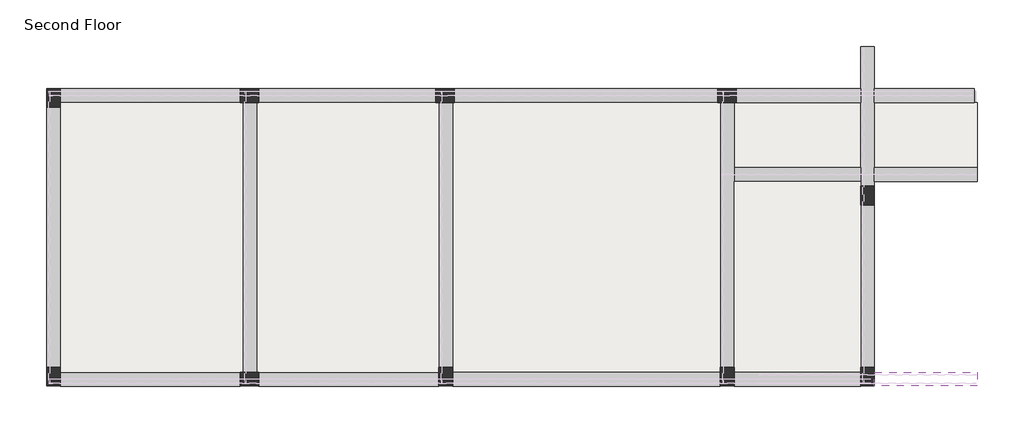
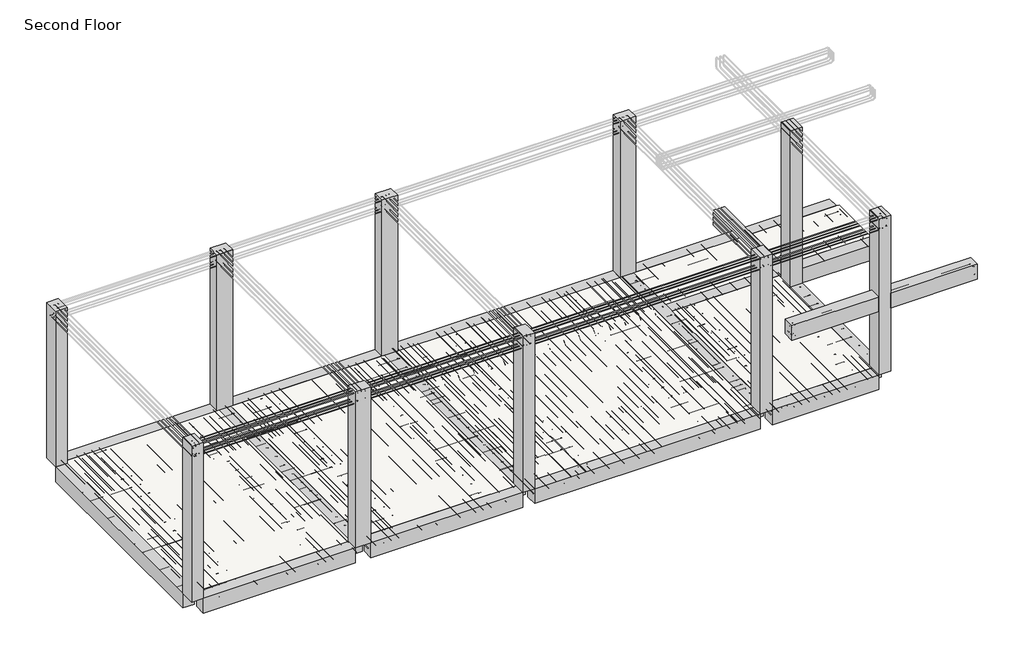
# One storey, part 1 of 4: 10 columns, 9 beams, 5 slabs.
"""IFC4 building model written with IfcOpenShell, lengths in millimetres."""

from ifc_helpers import new_model, si_unit, frame, origin, place, context, project, spatial, polyline, outline, extrude, faceted_brep, element, save

model = new_model("IFC4")

# Units and contexts
model_context = context("Model", 3, world=origin())
ifc_project = project(units=[si_unit("LENGTHUNIT", "METRE", prefix="MILLI")], contexts=[model_context])

# Site, building, storey
site = spatial("IfcSite", under=ifc_project)
building = spatial("IfcBuilding", under=site)
storey = spatial("IfcBuildingStorey", under=building, Name="Second Floor", Elevation=6400.8)

# Beams
placement = place(None, origin())
element("IfcBeam", 1, ObjectType="M_Concrete-Rectangular Beam : 9\" X12\"", at=placement, inside=storey, context=model_context, shape_type="Brep", body=[
    faceted_brep([(3956.0882476, 186.4334631, 6400.8), (3956.0882476, 415.0334631, 6400.8), (1885.9882476, 415.0334631, 6400.8), (1885.9882476, 186.4334631, 6400.8), (3956.0882476, 186.4334631, 6096.0), (1885.9882476, 186.4334631, 6096.0), (3956.0882476, 415.0334631, 6096.0), (1885.9882476, 415.0334631, 6096.0), (3956.0882476, 415.0334631, 6248.4), (1885.9882476, 415.0334631, 6248.4)], [[[0, 1, 2, 3]], [[4, 0, 3, 5]], [[6, 4, 5, 7]], [[1, 8, 6, 7, 9, 2]], [[1, 0, 4, 6, 8]], [[3, 2, 9, 7, 5]]]),
    faceted_brep([(-9150.3117524, 186.4334631, 6400.8), (-9150.3117524, 415.0334631, 6400.8), (-9150.3117524, 415.0334631, 6248.4), (-9150.3117524, 415.0334631, 6096.0), (-9150.3117524, 186.4334631, 6096.0), (-6203.9117524, 415.0334631, 6400.8), (-6203.9117524, 186.4334631, 6400.8), (-6203.9117524, 186.4334631, 6096.0), (-6203.9117524, 415.0334631, 6096.0)], [[[0, 1, 2, 3, 4]], [[5, 6, 7, 8]], [[1, 0, 6, 5]], [[0, 4, 7, 6]], [[4, 3, 8, 7]], [[3, 2, 1, 5, 8]]]),
    faceted_brep([(-5899.1117524, 186.4334631, 6400.8), (-5899.1117524, 415.0334631, 6400.8), (-5899.1117524, 415.0334631, 6096.0), (-5899.1117524, 186.4334631, 6096.0), (-2952.7117524, 415.0334631, 6400.8), (-2952.7117524, 186.4334631, 6400.8), (-2952.7117524, 186.4334631, 6096.0), (-2952.7117524, 415.0334631, 6096.0), (-2952.7117524, 415.0334631, 6248.4)], [[[0, 1, 2, 3]], [[4, 5, 6, 7, 8]], [[1, 0, 5, 4]], [[0, 3, 6, 5]], [[3, 2, 7, 6]], [[2, 1, 4, 8, 7]]]),
    faceted_brep([(-2724.1117524, 186.4334631, 6400.8), (-2724.1117524, 415.0334631, 6400.8), (-2724.1117524, 415.0334631, 6248.4), (-2724.1117524, 415.0334631, 6096.0), (-2724.1117524, 186.4334631, 6096.0), (1657.3882476, 415.0334631, 6400.8), (1657.3882476, 186.4334631, 6400.8), (1657.3882476, 186.4334631, 6096.0), (1657.3882476, 415.0334631, 6096.0), (1657.3882476, 415.0334631, 6248.4)], [[[0, 1, 2, 3, 4]], [[5, 6, 7, 8, 9]], [[1, 0, 6, 5]], [[0, 4, 7, 6]], [[4, 3, 8, 7]], [[3, 2, 1, 5, 9, 8]]]),
])
element("IfcBeam", 2, ObjectType="M_Concrete-Rectangular Beam : 9\" X12\"", at=placement, inside=storey, context=model_context, shape_type="Brep", body=[
    faceted_brep([(3956.0882476, 5755.7334631, 6400.8), (4184.6882476, 5755.7334631, 6400.8), (4184.6882476, 5755.7334631, 6096.0), (3956.0882476, 5755.7334631, 6096.0), (3956.0882476, 5063.2334631, 6400.8), (3956.0882476, 4834.6334631, 6400.8), (3956.0882476, 3767.8334631, 6400.8), (3956.0882476, 3539.2334631, 6400.8), (3956.0882476, 3463.0334631, 6400.8), (4184.6882476, 3463.0334631, 6400.8), (4184.6882476, 3539.2334631, 6400.8), (4184.6882476, 3767.8334631, 6400.8), (4184.6882476, 4834.6334631, 6400.8), (4184.6882476, 5063.2334631, 6400.8), (4184.6882476, 3463.0334631, 6096.0), (4184.6882476, 3539.2334631, 6096.0), (4184.6882476, 3767.8334631, 6096.0), (4184.6882476, 4834.6334631, 6096.0), (4184.6882476, 5063.2334631, 6096.0), (3956.0882476, 3463.0334631, 6096.0), (3956.0882476, 3539.2334631, 6096.0), (3956.0882476, 3767.8334631, 6096.0), (3956.0882476, 4834.6334631, 6096.0), (3956.0882476, 5063.2334631, 6096.0)], [[[0, 1, 2, 3]], [[1, 0, 4, 5, 6, 7, 8, 9, 10, 11, 12, 13]], [[2, 1, 13, 12, 11, 10, 9, 14, 15, 16, 17, 18]], [[3, 2, 18, 17, 16, 15, 14, 19, 20, 21, 22, 23]], [[0, 3, 23, 22, 21, 20, 19, 8, 7, 6, 5, 4]], [[9, 8, 19, 14]]]),
    faceted_brep([(4184.6882476, 491.2334631, 6400.8), (3956.0882476, 491.2334631, 6400.8), (3956.0882476, 491.2334631, 6096.0), (4184.6882476, 491.2334631, 6096.0), (3956.0882476, 3158.2334631, 6400.8), (4184.6882476, 3158.2334631, 6400.8), (4184.6882476, 3158.2334631, 6096.0), (3956.0882476, 3158.2334631, 6096.0)], [[[0, 1, 2, 3]], [[4, 5, 6, 7]], [[1, 0, 5, 4]], [[0, 3, 6, 5]], [[3, 2, 7, 6]], [[2, 1, 4, 7]]]),
])
element("IfcBeam", 3, ObjectType="M_Concrete-Rectangular Beam : 9\" X12\"", at=placement, inside=storey, context=model_context, shape_type="Brep", body=[
    faceted_brep([(5815.3882476, 4834.6334631, 6400.8), (5815.3882476, 4834.6334631, 6096.0), (5815.3882476, 5063.2334631, 6096.0), (5815.3882476, 5063.2334631, 6400.8), (4184.6882476, 4834.6334631, 6400.8), (4184.6882476, 5063.2334631, 6400.8), (4184.6882476, 5063.2334631, 6096.0), (4184.6882476, 4834.6334631, 6096.0), (4184.6882476, 4834.6334631, 6248.4)], [[[0, 1, 2, 3]], [[4, 5, 6, 7, 8]], [[0, 3, 5, 4]], [[3, 2, 6, 5]], [[2, 1, 7, 6]], [[1, 0, 4, 8, 7]]]),
    faceted_brep([(3956.0882476, 4834.6334631, 6400.8), (3956.0882476, 5063.2334631, 6400.8), (1924.0882476, 5063.2334631, 6400.8), (1924.0882476, 4834.6334631, 6400.8), (1924.0882476, 5063.2334631, 6096.0), (3956.0882476, 5063.2334631, 6096.0), (3956.0882476, 4834.6334631, 6096.0), (1924.0882476, 4834.6334631, 6096.0), (3956.0882476, 4834.6334631, 6248.4)], [[[0, 1, 2, 3]], [[4, 2, 1, 5]], [[5, 6, 7, 4]], [[6, 8, 0, 3, 7]], [[1, 0, 8, 6, 5]], [[3, 2, 4, 7]]]),
    faceted_brep([(-9150.3117524, 4834.6334631, 6400.8), (-9150.3117524, 5063.2334631, 6400.8), (-9150.3117524, 5063.2334631, 6096.0), (-9150.3117524, 4834.6334631, 6096.0), (-9150.3117524, 4834.6334631, 6248.4), (-6203.9117524, 5063.2334631, 6400.8), (-6203.9117524, 4834.6334631, 6400.8), (-6203.9117524, 4834.6334631, 6096.0), (-6203.9117524, 5063.2334631, 6096.0)], [[[0, 1, 2, 3, 4]], [[5, 6, 7, 8]], [[1, 0, 6, 5]], [[2, 1, 5, 8]], [[3, 2, 8, 7]], [[0, 4, 3, 7, 6]]]),
    faceted_brep([(1619.2882476, 5063.2334631, 6400.8), (1619.2882476, 4834.6334631, 6400.8), (1619.2882476, 4834.6334631, 6096.0), (1619.2882476, 5063.2334631, 6096.0), (-2698.7117524, 4834.6334631, 6400.8), (-2698.7117524, 5063.2334631, 6400.8), (-2698.7117524, 5063.2334631, 6096.0), (-2698.7117524, 4834.6334631, 6096.0)], [[[0, 1, 2, 3]], [[4, 5, 6, 7]], [[1, 0, 5, 4]], [[0, 3, 6, 5]], [[3, 2, 7, 6]], [[2, 1, 4, 7]]]),
    faceted_brep([(-3003.5117524, 4834.6334631, 6400.8), (-3003.5117524, 5063.2334631, 6400.8), (-5899.1117524, 5063.2334631, 6400.8), (-5899.1117524, 4834.6334631, 6400.8), (-3003.5117524, 5063.2334631, 6096.0), (-5899.1117524, 5063.2334631, 6096.0), (-3003.5117524, 4834.6334631, 6096.0), (-5899.1117524, 4834.6334631, 6096.0)], [[[0, 1, 2, 3]], [[1, 4, 5, 2]], [[4, 6, 7, 5]], [[6, 0, 3, 7]], [[1, 0, 6, 4]], [[3, 2, 5, 7]]]),
])
element("IfcBeam", 4, ObjectType="M_Concrete-Rectangular Beam : 9\" X12\"", at=placement, inside=storey, context=model_context, shape_type="SweptSolid", body=[
    extrude(outline(polyline([(-9378.9117524, 4758.4334631), (-9150.3117524, 4758.4334631), (-9150.3117524, 491.2334631), (-9378.9117524, 491.2334631), (-9378.9117524, 4758.4334631)])), frame((0.0, 0.0, 6096.0), z_axis=(0.0, 0.0, 1.0), x_axis=(1.0, 0.0, 0.0)), (0.0, 0.0, 1.0), 304.8),
])
element("IfcBeam", 5, ObjectType="M_Concrete-Rectangular Beam : 9\" X12\"", at=placement, inside=storey, context=model_context, shape_type="Brep", body=[
    faceted_brep([(-6165.8117524, 415.0334631, 6400.8), (-5937.2117524, 415.0334631, 6400.8), (-5937.2117524, 4834.6334631, 6400.8), (-6165.8117524, 4834.6334631, 6400.8), (-5937.2117524, 415.0334631, 6248.4), (-5937.2117524, 415.0334631, 6096.0), (-5937.2117524, 4834.6334631, 6096.0), (-5937.2117524, 4834.6334631, 6248.4), (-6165.8117524, 415.0334631, 6096.0), (-6165.8117524, 4834.6334631, 6096.0), (-6165.8117524, 415.0334631, 6248.4), (-6165.8117524, 4834.6334631, 6248.4)], [[[0, 1, 2, 3]], [[1, 4, 5, 6, 7, 2]], [[5, 8, 9, 6]], [[8, 10, 0, 3, 11, 9]], [[1, 0, 10, 8, 5, 4]], [[3, 2, 7, 6, 9, 11]]]),
])
element("IfcBeam", 6, ObjectType="M_Concrete-Rectangular Beam : 9\" X12\"", at=placement, inside=storey, context=model_context, shape_type="Brep", body=[
    faceted_brep([(-2952.7117524, 491.2334631, 6400.8), (-2724.1117524, 491.2334631, 6400.8), (-2724.1117524, 4834.6334631, 6400.8), (-2952.7117524, 4834.6334631, 6400.8), (-2724.1117524, 491.2334631, 6096.0), (-2724.1117524, 4834.6334631, 6096.0), (-2724.1117524, 4834.6334631, 6248.4), (-2952.7117524, 491.2334631, 6096.0), (-2952.7117524, 4834.6334631, 6096.0), (-2952.7117524, 4834.6334631, 6248.4)], [[[0, 1, 2, 3]], [[1, 4, 5, 6, 2]], [[4, 7, 8, 5]], [[7, 0, 3, 9, 8]], [[1, 0, 7, 4]], [[3, 2, 6, 5, 8, 9]]]),
])
element("IfcBeam", 7, ObjectType="M_Concrete-Rectangular Beam : 9\" X12\"", at=placement, inside=storey, context=model_context, shape_type="Brep", body=[
    faceted_brep([(1657.3882476, 491.2334631, 6400.8), (1885.9882476, 491.2334631, 6400.8), (1885.9882476, 3539.2334631, 6400.8), (1885.9882476, 3767.8334631, 6400.8), (1885.9882476, 4834.6334631, 6400.8), (1657.3882476, 4834.6334631, 6400.8), (1885.9882476, 491.2334631, 6096.0), (1885.9882476, 3539.2334631, 6096.0), (1885.9882476, 3767.8334631, 6096.0), (1885.9882476, 4834.6334631, 6096.0), (1885.9882476, 4834.6334631, 6248.4), (1657.3882476, 491.2334631, 6096.0), (1657.3882476, 4834.6334631, 6096.0), (1657.3882476, 4834.6334631, 6248.4)], [[[0, 1, 2, 3, 4, 5]], [[1, 6, 7, 8, 9, 10, 4, 3, 2]], [[6, 11, 12, 9, 8, 7]], [[11, 0, 5, 13, 12]], [[1, 0, 11, 6]], [[5, 4, 10, 9, 12, 13]]]),
])
element("IfcBeam", 8, ObjectType="M_Concrete-Rectangular Beam : 9\" X12\"", at=placement, inside=storey, context=model_context, shape_type="Brep", body=[
    faceted_brep([(5871.6882476, 3539.2334631, 6400.8), (5871.6882476, 3539.2334631, 6096.0), (5871.6882476, 3767.8334631, 6096.0), (5871.6882476, 3767.8334631, 6248.4), (5871.6882476, 3767.8334631, 6400.8), (4184.6882476, 3539.2334631, 6400.8), (4184.6882476, 3767.8334631, 6400.8), (4184.6882476, 3767.8334631, 6248.4), (4184.6882476, 3767.8334631, 6096.0), (4184.6882476, 3539.2334631, 6096.0)], [[[0, 1, 2, 3, 4]], [[5, 6, 7, 8, 9]], [[0, 4, 6, 5]], [[4, 3, 2, 8, 7, 6]], [[2, 1, 9, 8]], [[1, 0, 5, 9]]]),
    faceted_brep([(1885.9882476, 3767.8334631, 6400.8), (1885.9882476, 3539.2334631, 6400.8), (3956.0882476, 3539.2334631, 6400.8), (3956.0882476, 3767.8334631, 6400.8), (1885.9882476, 3767.8334631, 6096.0), (1885.9882476, 3767.8334631, 6248.4), (3956.0882476, 3767.8334631, 6248.4), (3956.0882476, 3767.8334631, 6096.0), (1885.9882476, 3539.2334631, 6096.0), (3956.0882476, 3539.2334631, 6096.0), (1885.9882476, 3539.2334631, 6248.4), (3956.0882476, 3539.2334631, 6248.4)], [[[0, 1, 2, 3]], [[4, 5, 0, 3, 6, 7]], [[8, 4, 7, 9]], [[1, 10, 8, 9, 11, 2]], [[1, 0, 5, 4, 8, 10]], [[3, 2, 11, 9, 7, 6]]]),
])
element("IfcBeam", 9, ObjectType="M_Concrete-Rectangular Beam : 9\" X12\"", at=placement, inside=storey, context=model_context, shape_type="SweptSolid", body=[
    extrude(outline(polyline([(2271.6882476, 186.4334631), (2271.6882476, 415.0334631), (3956.0882476, 415.0334631), (3956.0882476, 186.4334631), (2271.6882476, 186.4334631)])), frame((0.0, 0.0, 7696.2), z_axis=(0.0, 0.0, 1.0), x_axis=(1.0, 0.0, 0.0)), (0.0, 0.0, 1.0), 304.8),
    extrude(outline(polyline([(5871.6882476, 415.0334631), (5871.6882476, 186.4334631), (4184.6882476, 186.4334631), (4184.6882476, 415.0334631), (5871.6882476, 415.0334631)])), frame((0.0, 0.0, 7696.2), z_axis=(0.0, 0.0, 1.0), x_axis=(1.0, 0.0, 0.0)), (0.0, 0.0, 1.0), 304.8),
])

# Columns
element("IfcColumn", 10, ObjectType="M_Concrete-Rectangular-Column : 9\" x 12\"", at=placement, inside=storey, context=model_context, shape_type="SweptSolid", body=[
    extrude(outline(polyline([(-9150.3117524, 5063.2334631), (-9150.3117524, 4758.4334631), (-9378.9117524, 4758.4334631), (-9378.9117524, 5063.2334631), (-9150.3117524, 5063.2334631)])), frame((0.0, 0.0, 6400.8), z_axis=(0.0, 0.0, 1.0), x_axis=(1.0, 0.0, 0.0)), (0.0, 0.0, 1.0), 3200.4),
])
element("IfcColumn", 11, ObjectType="M_Concrete-Rectangular-Column : 9\" x 12\"", at=placement, inside=storey, context=model_context, shape_type="SweptSolid", body=[
    extrude(outline(polyline([(-9150.3117524, 491.2334631), (-9150.3117524, 186.4334631), (-9378.9117524, 186.4334631), (-9378.9117524, 491.2334631), (-9150.3117524, 491.2334631)])), frame((0.0, 0.0, 6400.8), z_axis=(0.0, 0.0, 1.0), x_axis=(1.0, 0.0, 0.0)), (0.0, 0.0, 1.0), 3200.4),
])
element("IfcColumn", 12, ObjectType="M_Concrete-Rectangular-Column : 9\" x 12\"", at=placement, inside=storey, context=model_context, shape_type="Brep", body=[
    faceted_brep([(-6203.9117524, 415.0334631, 6400.8), (-5899.1117524, 415.0334631, 6400.8), (-5899.1117524, 186.4334631, 6400.8), (-6203.9117524, 186.4334631, 6400.8), (-6203.9117524, 415.0334631, 9601.2), (-5899.1117524, 415.0334631, 9601.2), (-5899.1117524, 415.0334631, 9296.4), (-6203.9117524, 415.0334631, 9296.4), (-5899.1117524, 186.4334631, 9601.2), (-5899.1117524, 186.4334631, 9296.4), (-6203.9117524, 186.4334631, 9601.2), (-6203.9117524, 186.4334631, 9296.4)], [[[0, 1, 2, 3]], [[4, 5, 6, 1, 0, 7]], [[5, 8, 9, 2, 1, 6]], [[8, 10, 11, 3, 2, 9]], [[10, 4, 7, 0, 3, 11]], [[4, 10, 8, 5]]]),
])
element("IfcColumn", 13, ObjectType="M_Concrete-Rectangular-Column : 9\" x 12\"", at=placement, inside=storey, context=model_context, shape_type="Brep", body=[
    faceted_brep([(-2952.7117524, 186.4334631, 6400.8), (-2952.7117524, 491.2334631, 6400.8), (-2724.1117524, 491.2334631, 6400.8), (-2724.1117524, 186.4334631, 6400.8), (-2952.7117524, 186.4334631, 9601.2), (-2952.7117524, 415.0334631, 9601.2), (-2952.7117524, 491.2334631, 9601.2), (-2952.7117524, 186.4334631, 9296.4), (-2724.1117524, 491.2334631, 9601.2), (-2724.1117524, 415.0334631, 9601.2), (-2724.1117524, 186.4334631, 9601.2), (-2724.1117524, 186.4334631, 9296.4)], [[[0, 1, 2, 3]], [[4, 5, 6, 1, 0, 7]], [[6, 8, 2, 1]], [[8, 9, 10, 11, 3, 2]], [[10, 4, 7, 0, 3, 11]], [[4, 10, 9, 8, 6, 5]]]),
])
element("IfcColumn", 14, ObjectType="M_Concrete-Rectangular-Column : 9\" x 12\"", at=placement, inside=storey, context=model_context, shape_type="Brep", body=[
    faceted_brep([(1657.3882476, 186.4334631, 6400.8), (1657.3882476, 491.2334631, 6400.8), (1885.9882476, 491.2334631, 6400.8), (1885.9882476, 186.4334631, 6400.8), (1657.3882476, 186.4334631, 9601.2), (1657.3882476, 415.0334631, 9601.2), (1657.3882476, 491.2334631, 9601.2), (1657.3882476, 186.4334631, 9296.4), (1885.9882476, 491.2334631, 9601.2), (1885.9882476, 415.0334631, 9601.2), (1885.9882476, 186.4334631, 9601.2), (1885.9882476, 186.4334631, 9296.4)], [[[0, 1, 2, 3]], [[4, 5, 6, 1, 0, 7]], [[6, 8, 2, 1]], [[8, 9, 10, 11, 3, 2]], [[10, 4, 7, 0, 3, 11]], [[4, 10, 9, 8, 6, 5]]]),
])
element("IfcColumn", 15, ObjectType="M_Concrete-Rectangular-Column : 9\" x 12\"", at=placement, inside=storey, context=model_context, shape_type="Brep", body=[
    faceted_brep([(3956.0882476, 186.4334631, 6400.8), (3956.0882476, 491.2334631, 6400.8), (4184.6882476, 491.2334631, 6400.8), (4184.6882476, 186.4334631, 6400.8), (3956.0882476, 186.4334631, 9601.2), (3956.0882476, 491.2334631, 9601.2), (3956.0882476, 186.4334631, 7696.2), (3956.0882476, 186.4334631, 8001.0), (4184.6882476, 491.2334631, 9601.2), (4184.6882476, 186.4334631, 9601.2), (4184.6882476, 186.4334631, 8001.0), (4184.6882476, 186.4334631, 7696.2)], [[[0, 1, 2, 3]], [[4, 5, 1, 0, 6, 7]], [[5, 8, 2, 1]], [[8, 9, 10, 11, 3, 2]], [[9, 4, 7, 6, 0, 3, 11, 10]], [[4, 9, 8, 5]]]),
])
element("IfcColumn", 16, ObjectType="M_Concrete-Rectangular-Column : 9\" x 12\"", at=placement, inside=storey, context=model_context, shape_type="Brep", body=[
    faceted_brep([(3956.0882476, 3158.2334631, 6400.8), (3956.0882476, 3463.0334631, 6400.8), (4184.6882476, 3463.0334631, 6400.8), (4184.6882476, 3158.2334631, 6400.8), (3956.0882476, 3158.2334631, 9601.2), (3956.0882476, 3463.0334631, 9601.2), (3956.0882476, 3463.0334631, 9296.4), (3956.0882476, 3158.2334631, 9296.4), (4184.6882476, 3463.0334631, 9601.2), (4184.6882476, 3463.0334631, 9296.4), (4184.6882476, 3158.2334631, 9601.2), (4184.6882476, 3158.2334631, 9296.4)], [[[0, 1, 2, 3]], [[4, 5, 6, 1, 0, 7]], [[5, 8, 9, 2, 1, 6]], [[8, 10, 11, 3, 2, 9]], [[10, 4, 7, 0, 3, 11]], [[4, 10, 8, 5]]]),
])
element("IfcColumn", 17, ObjectType="M_Concrete-Rectangular-Column : 9\" x 12\"", at=placement, inside=storey, context=model_context, shape_type="Brep", body=[
    faceted_brep([(1924.0882476, 4834.6334631, 6400.8), (1619.2882476, 4834.6334631, 6400.8), (1619.2882476, 5063.2334631, 6400.8), (1924.0882476, 5063.2334631, 6400.8), (1924.0882476, 4834.6334631, 9601.2), (1619.2882476, 4834.6334631, 9601.2), (1619.2882476, 4834.6334631, 9296.4), (1924.0882476, 4834.6334631, 9296.4), (1619.2882476, 5063.2334631, 9601.2), (1619.2882476, 5063.2334631, 9296.4), (1924.0882476, 5063.2334631, 9601.2), (1924.0882476, 5063.2334631, 9296.4)], [[[0, 1, 2, 3]], [[4, 5, 6, 1, 0, 7]], [[5, 8, 9, 2, 1, 6]], [[8, 10, 11, 3, 2, 9]], [[10, 4, 7, 0, 3, 11]], [[4, 10, 8, 5]]]),
])
element("IfcColumn", 18, ObjectType="M_Concrete-Rectangular-Column : 9\" x 12\"", at=placement, inside=storey, context=model_context, shape_type="Brep", body=[
    faceted_brep([(-2698.7117524, 4834.6334631, 6400.8), (-3003.5117524, 4834.6334631, 6400.8), (-3003.5117524, 5063.2334631, 6400.8), (-2698.7117524, 5063.2334631, 6400.8), (-2698.7117524, 4834.6334631, 9601.2), (-3003.5117524, 4834.6334631, 9601.2), (-3003.5117524, 4834.6334631, 9296.4), (-2698.7117524, 4834.6334631, 9296.4), (-3003.5117524, 5063.2334631, 9601.2), (-3003.5117524, 5063.2334631, 9296.4), (-2698.7117524, 5063.2334631, 9601.2), (-2698.7117524, 5063.2334631, 9296.4)], [[[0, 1, 2, 3]], [[4, 5, 6, 1, 0, 7]], [[5, 8, 9, 2, 1, 6]], [[8, 10, 11, 3, 2, 9]], [[10, 4, 7, 0, 3, 11]], [[4, 10, 8, 5]]]),
])
element("IfcColumn", 19, ObjectType="M_Concrete-Rectangular-Column : 9\" x 12\"", at=placement, inside=storey, context=model_context, shape_type="Brep", body=[
    faceted_brep([(-5899.1117524, 4834.6334631, 6400.8), (-6203.9117524, 4834.6334631, 6400.8), (-6203.9117524, 5063.2334631, 6400.8), (-5899.1117524, 5063.2334631, 6400.8), (-5899.1117524, 4834.6334631, 9601.2), (-6203.9117524, 4834.6334631, 9601.2), (-6203.9117524, 4834.6334631, 9296.4), (-5899.1117524, 4834.6334631, 9296.4), (-6203.9117524, 5063.2334631, 9601.2), (-6203.9117524, 5063.2334631, 9296.4), (-5899.1117524, 5063.2334631, 9601.2), (-5899.1117524, 5063.2334631, 9296.4)], [[[0, 1, 2, 3]], [[4, 5, 6, 1, 0, 7]], [[5, 8, 9, 2, 1, 6]], [[8, 10, 11, 3, 2, 9]], [[10, 4, 7, 0, 3, 11]], [[4, 10, 8, 5]]]),
])

# Slabs
element("IfcSlab", 20, ObjectType="FLOOR SLAB 6\"", at=placement, inside=storey, context=model_context, shape_type="Brep", body=[
    faceted_brep([(-6165.8117524, 4834.6334631, 6248.4), (-6165.8117524, 415.0334631, 6248.4), (-9150.3117524, 415.0334631, 6248.4), (-9150.3117524, 4834.6334631, 6248.4), (-6165.8117524, 4834.6334631, 6400.8), (-6203.9117524, 4834.6334631, 6400.8), (-9150.3117524, 4834.6334631, 6400.8), (-9150.3117524, 4758.4334631, 6400.8), (-9150.3117524, 491.2334631, 6400.8), (-9150.3117524, 415.0334631, 6400.8), (-6203.9117524, 415.0334631, 6400.8), (-6165.8117524, 415.0334631, 6400.8)], [[[0, 1, 2, 3]], [[4, 5, 6, 7, 8, 9, 10, 11]], [[1, 0, 4, 11]], [[2, 1, 11, 10, 9]], [[3, 2, 9, 8, 7, 6]], [[0, 3, 6, 5, 4]]]),
])
element("IfcSlab", 21, ObjectType="FLOOR SLAB 6\"", at=placement, inside=storey, context=model_context, shape_type="Brep", body=[
    faceted_brep([(-2952.7117524, 4834.6334631, 6248.4), (-2952.7117524, 415.0334631, 6248.4), (-5937.2117524, 415.0334631, 6248.4), (-5937.2117524, 4834.6334631, 6248.4), (-2952.7117524, 4834.6334631, 6400.8), (-3003.5117524, 4834.6334631, 6400.8), (-5899.1117524, 4834.6334631, 6400.8), (-5937.2117524, 4834.6334631, 6400.8), (-5937.2117524, 415.0334631, 6400.8), (-5899.1117524, 415.0334631, 6400.8), (-2952.7117524, 415.0334631, 6400.8), (-2952.7117524, 491.2334631, 6400.8)], [[[0, 1, 2, 3]], [[4, 5, 6, 7, 8, 9, 10, 11]], [[1, 0, 4, 11, 10]], [[2, 1, 10, 9, 8]], [[3, 2, 8, 7]], [[0, 3, 7, 6, 5, 4]]]),
])
element("IfcSlab", 22, ObjectType="FLOOR SLAB 6\"", at=placement, inside=storey, context=model_context, shape_type="Brep", body=[
    faceted_brep([(1657.3882476, 4834.6334631, 6248.4), (1657.3882476, 415.0334631, 6248.4), (-2724.1117524, 415.0334631, 6248.4), (-2724.1117524, 4834.6334631, 6248.4), (1657.3882476, 4834.6334631, 6400.8), (1619.2882476, 4834.6334631, 6400.8), (-2698.7117524, 4834.6334631, 6400.8), (-2724.1117524, 4834.6334631, 6400.8), (-2724.1117524, 491.2334631, 6400.8), (-2724.1117524, 415.0334631, 6400.8), (1657.3882476, 415.0334631, 6400.8), (1657.3882476, 491.2334631, 6400.8)], [[[0, 1, 2, 3]], [[4, 5, 6, 7, 8, 9, 10, 11]], [[1, 0, 4, 11, 10]], [[2, 1, 10, 9]], [[3, 2, 9, 8, 7]], [[0, 3, 7, 6, 5, 4]]]),
])
element("IfcSlab", 23, ObjectType="FLOOR SLAB 6\"", at=placement, inside=storey, context=model_context, shape_type="Brep", body=[
    faceted_brep([(3956.0882476, 415.0334631, 6248.4), (1885.9882476, 415.0334631, 6248.4), (1885.9882476, 3539.2334631, 6248.4), (3956.0882476, 3539.2334631, 6248.4), (3956.0882476, 415.0334631, 6400.8), (3956.0882476, 491.2334631, 6400.8), (3956.0882476, 3158.2334631, 6400.8), (3956.0882476, 3463.0334631, 6400.8), (3956.0882476, 3539.2334631, 6400.8), (1885.9882476, 3539.2334631, 6400.8), (1885.9882476, 491.2334631, 6400.8), (1885.9882476, 415.0334631, 6400.8)], [[[0, 1, 2, 3]], [[4, 5, 6, 7, 8, 9, 10, 11]], [[1, 0, 4, 11]], [[2, 1, 11, 10, 9]], [[3, 2, 9, 8]], [[0, 3, 8, 7, 6, 5, 4]]]),
])
element("IfcSlab", 24, ObjectType="FLOOR SLAB 6\"", at=placement, inside=storey, context=model_context, shape_type="Brep", body=[
    faceted_brep([(3956.0882476, 3767.8334631, 6248.4), (1885.9882476, 3767.8334631, 6248.4), (1885.9882476, 4834.6334631, 6248.4), (3956.0882476, 4834.6334631, 6248.4), (3956.0882476, 3767.8334631, 6400.8), (3956.0882476, 4834.6334631, 6400.8), (1924.0882476, 4834.6334631, 6400.8), (1885.9882476, 4834.6334631, 6400.8), (1885.9882476, 3767.8334631, 6400.8)], [[[0, 1, 2, 3]], [[4, 5, 6, 7, 8]], [[1, 0, 4, 8]], [[2, 1, 8, 7]], [[3, 2, 7, 6, 5]], [[0, 3, 5, 4]]]),
    faceted_brep([(5871.6882476, 4834.6334631, 6248.4), (5871.6882476, 3767.8334631, 6248.4), (4184.6882476, 3767.8334631, 6248.4), (4184.6882476, 4834.6334631, 6248.4), (5871.6882476, 4834.6334631, 6400.8), (5815.3882476, 4834.6334631, 6400.8), (4184.6882476, 4834.6334631, 6400.8), (4184.6882476, 3767.8334631, 6400.8), (5871.6882476, 3767.8334631, 6400.8)], [[[0, 1, 2, 3]], [[4, 5, 6, 7, 8]], [[1, 0, 4, 8]], [[2, 1, 8, 7]], [[3, 2, 7, 6]], [[0, 3, 6, 5, 4]]]),
])

save(model, "model.ifc")

# Revit data of these elements
# Type "M_Concrete-Rectangular Beam : 9\" X12\""
#   Length [instance default] = 5' - 0"
#   b = 0' - 9"
#   h = 1' - 0"
#   Structural Material [instance default] = Concrete, Cast-in-Place gray
#   Assembly Code = ""
# Type "M_Concrete-Rectangular-Column : 9\" x 12\""
#   b = 0' - 9"
#   h = 1' - 0"
#   Structural Material [instance default] = Concrete, Cast-in-Place gray
# Type "FLOOR SLAB 6\""
#   Layers, outside or top first: 0' - 6" "Concrete, Cast-in-Place gray" (function 1)
# Elements 1, 2, 3, 4, 5, 6, 7, 8, 9 (IfcBeam, "M_Concrete-Rectangular Beam : 9\" X12\"")
#   Structural Material = Concrete, Cast-in-Place gray
#   Phase Created = New Construction
#   Materials on its faces: "Concrete, Cast-in-Place gray"
# Elements 10, 11, 12, 13, 14, 15, 16, 17, 18, 19 (IfcColumn, "M_Concrete-Rectangular-Column : 9\" x 12\"")
#   Structural Material = Concrete, Cast-in-Place gray
#   Phase Created = New Construction
#   Materials on its faces: "Concrete, Cast-in-Place gray"
# Elements 20, 21, 22, 23, 24 (IfcSlab, "FLOOR SLAB 6\"")
#   Height Offset From Level = 0' - 0"
#   built-in parameter 1001954 = 1
#   Phase Created = New Construction
#   Materials on its faces: "Concrete, Cast-in-Place gray"
# Materials
#   "Concrete, Cast-in-Place gray": class "Concrete", colour RGB 192 192 192, transparency 0, Description = "Cast-in-place concrete", Cost = 0
